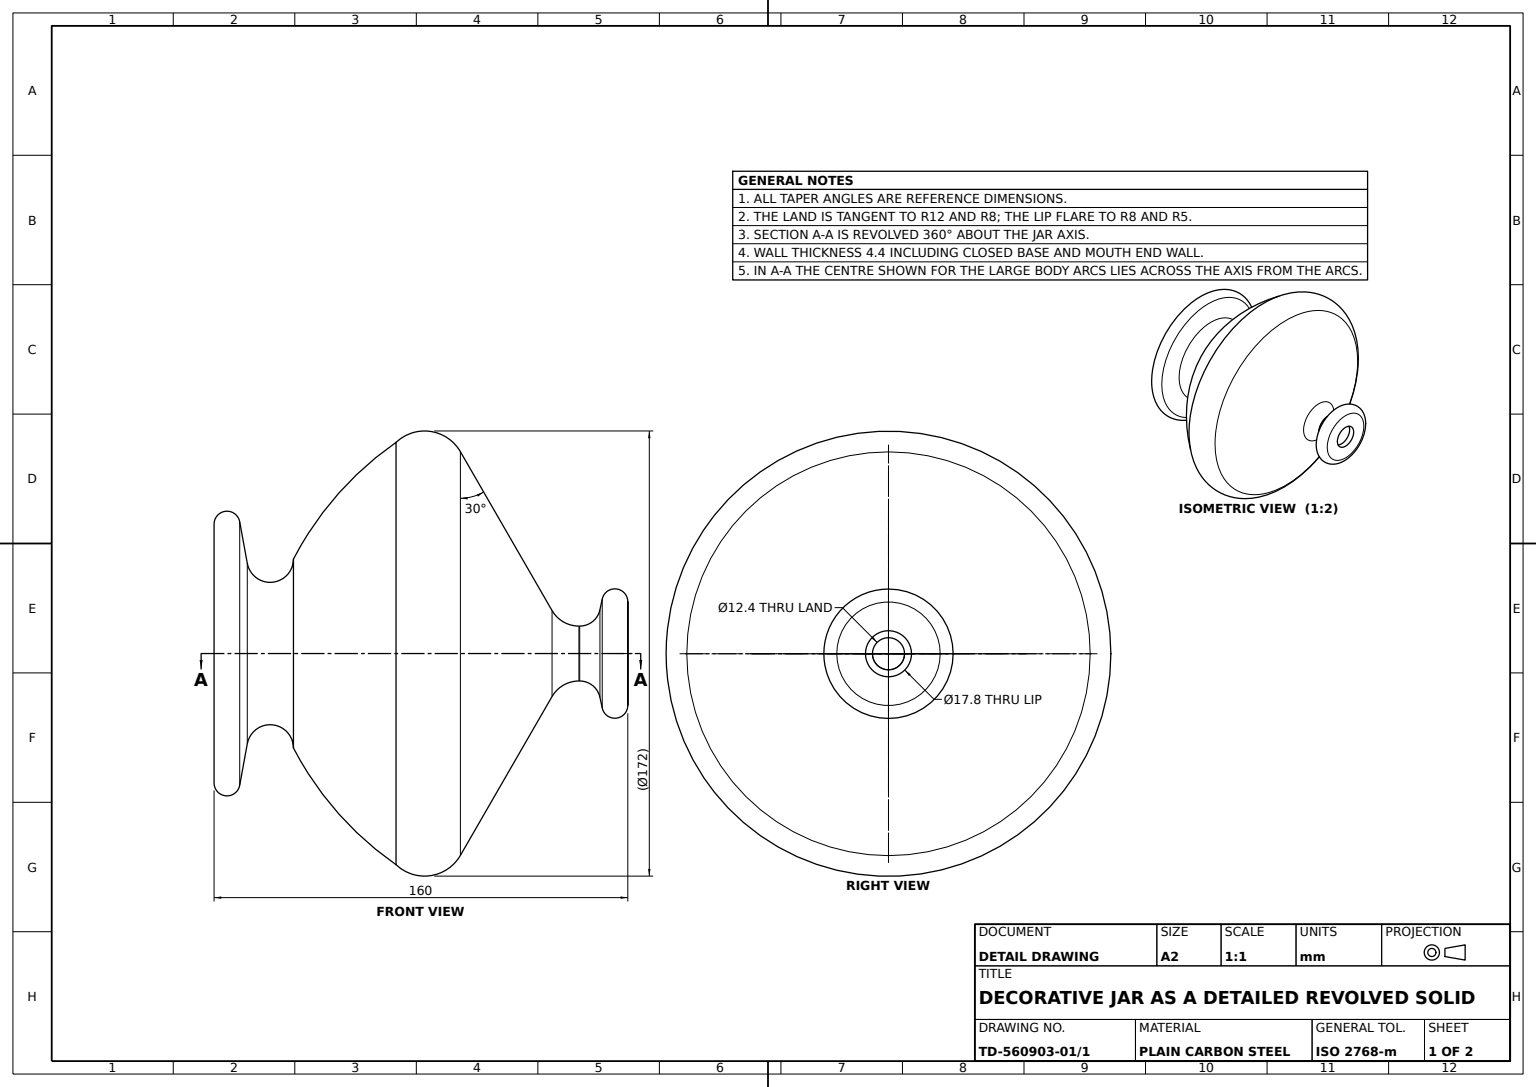
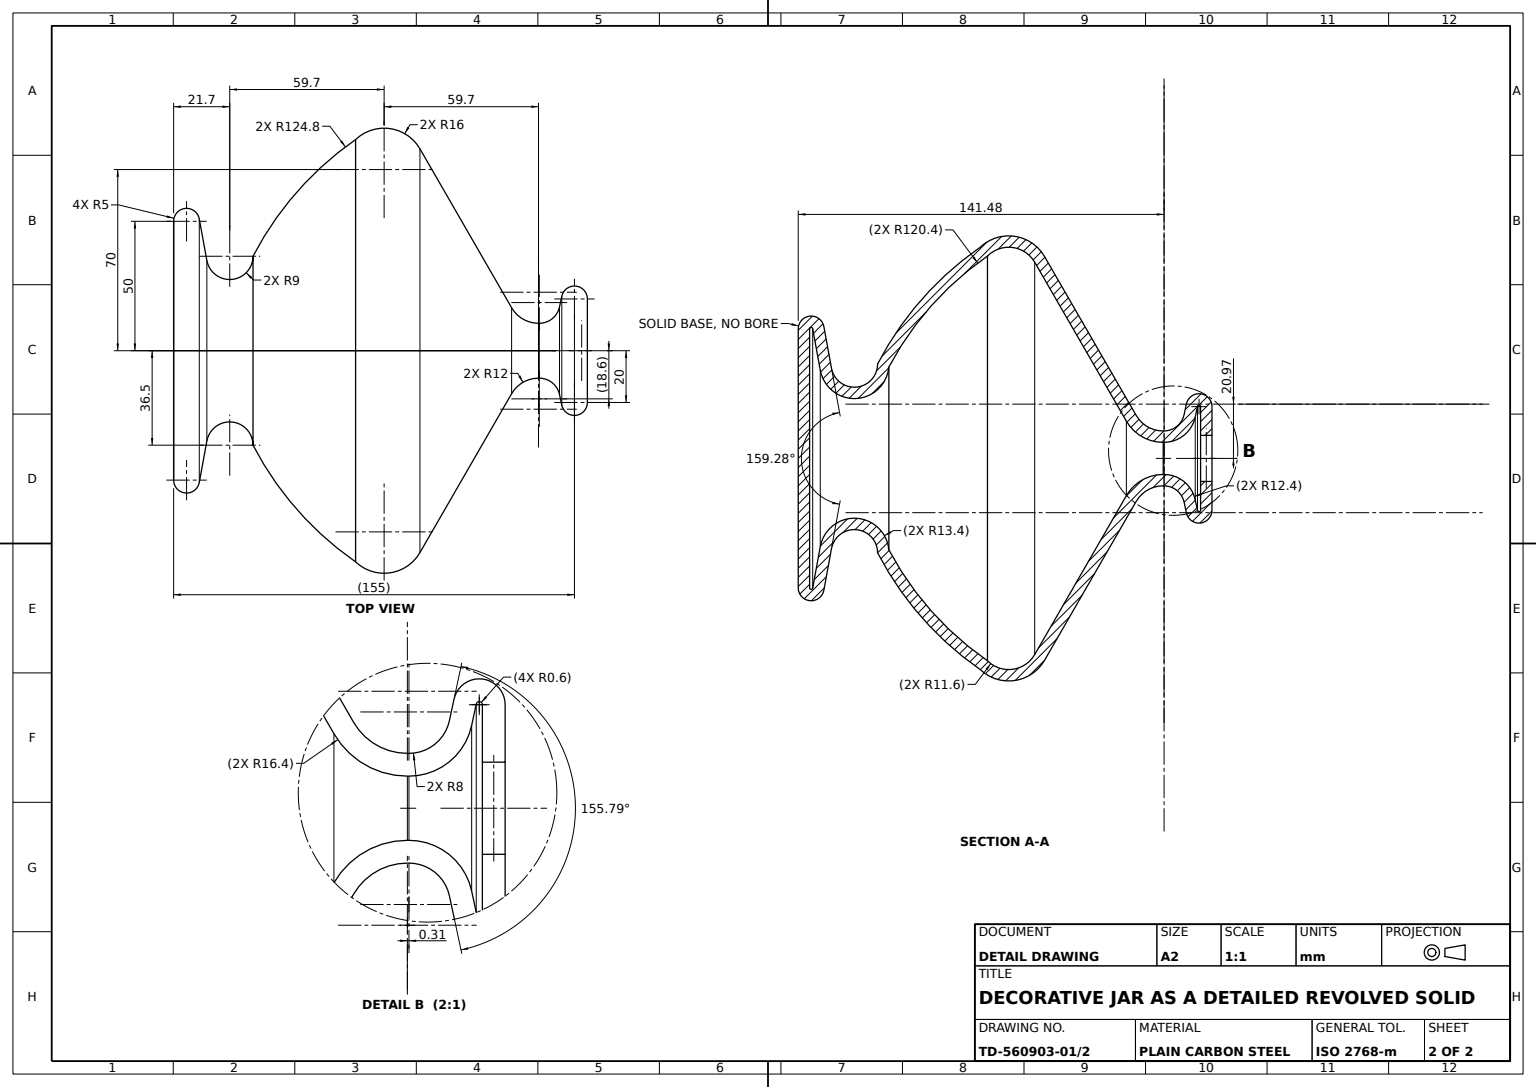
SolidWorks part; units mm, degrees
material "Plain Carbon Steel"
ref_plane "Front Plane" through (0, 0, 0) normal (0, 0, 1) x (1, 0, 0)
ref_plane "Top Plane" through (0, 0, 0) normal (0, 1, 0) x (1, 0, 0)
ref_plane "Right Plane" through (0, 0, 0) normal (1, 0, 0) x (0, 0, -1)
sketch "Jar Profile Sketch" plane through (0, 0, 0) normal (0, 0, 1) x (1, 0, 0)
  line L0 (-82.6187, 0) -> (85.3537, 0) construction
  line L1 (0, 194.5407) -> (0, -62.111) construction
  line L2 (0, 0) -> (-50, 0)
  line L3 (-34.8815, 12.8467) -> (-50.8992, 9.9185)
  line L4 (-78, 95.2564) -> (-16.6, 130.7057)
  line L5 (-10.6, 141.098) -> (-10.6, 141.4039)
  line L6 (-8.9, 160) -> (-8.9, 155.6)
  line L7 (-20, 160) -> (-8.9, 160)
  line L8 (-16.9221, 149.226) -> (-21.0487, 150.1112)
  line L9 (0, 4.4) -> (-50, 4.4)
  line L10 (-34.0902, 8.5185) -> (-50.1079, 5.5902)
  line L11 (-75.8, 91.4459) -> (-14.4, 126.8952)
  line L12 (-6.2, 141.098) -> (-6.2, 141.4039)
  line L13 (-15.9992, 153.5281) -> (-20.1258, 154.4133)
  line L14 (-20, 155.6) -> (-8.9, 155.6)
  line L15 (0, 0) -> (0, 4.4)
  line L17 (-79.1094, 94.6159) -> (-16.6, 130.7057) construction
  line L18 (-76.9094, 90.8054) -> (-14.4, 126.8952) construction
  line L20 (-20, 160) -> (0, 160) construction
  line L21 (-20, 155.6) -> (0, 155.6) construction
  arc A0 (-50.8992, 9.9185) -> (-50, 0) centre (-50, 5) ccw
  arc A1 (-34.8815, 12.8467) -> (-36.5, 30.7) centre (-36.5, 21.7) ccw
  arc A2 (-78, 95.2564) -> (-81.5898, 70.3693) centre (-70, 81.4) ccw
  arc A3 (-36.5, 30.7) -> (-81.5898, 70.3693) centre (20.9683, 141.481) cw
  arc A4 (-16.6, 130.7057) -> (-10.6, 141.098) centre (-22.6, 141.098) ccw
  arc A5 (-20, 160) -> (-21.0487, 150.1112) centre (-20, 155) ccw
  arc A6 (-16.9221, 149.226) -> (-10.6, 141.4039) centre (-18.6, 141.4039) cw
  arc A7 (-50.1079, 5.5902) -> (-50, 4.4) centre (-50, 5) ccw
  arc A8 (-34.0902, 8.5185) -> (-35.3177, 35.0477) centre (-36.5, 21.7) ccw
  arc A9 (-35.3177, 35.0477) -> (-78.1815, 73.1766) centre (20.9683, 141.481) cw
  arc A10 (-75.8, 91.4459) -> (-78.1815, 73.1766) centre (-70, 81.4) ccw
  arc A11 (-14.4, 126.8952) -> (-6.2, 141.098) centre (-22.6, 141.098) ccw
  arc A12 (-15.9992, 153.5281) -> (-6.2, 141.4039) centre (-18.6, 141.4039) cw
  arc A13 (-20, 155.6) -> (-20.1258, 154.4133) centre (-20, 155) ccw
  point P21 (-10.6, 134.1698)
  point P29 (-10.6, 147.8698)
  dimension "D2" = 32
  dimension "D4" = 18
  dimension "D9" = 124.8
  dimension "D12" = 12
  dimension "D15" = 10
  dimension "D19" = 8
  dimension "D1" = 50
  dimension "D3" = 5
  dimension "D5" = 36.5
  dimension "D6" = 21.7
  dimension "D7" = 59.7
  dimension "D8" = 70
  dimension "D10" = 60
  dimension "D11" = 13.7
  dimension "D13" = 10.6
  dimension "D14" = 20.9683
  dimension "D16" = 20
  dimension "D17" = 8.9
  dimension "D18" = 155
  dimension "D20" = 4.4
revolve "Jar Body Revolve 360°" add sketch "Jar Profile Sketch" angle 360 about L1
